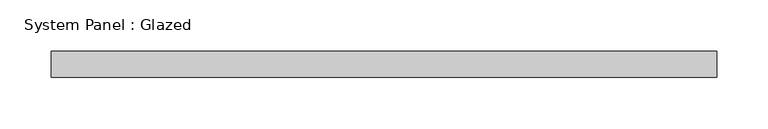
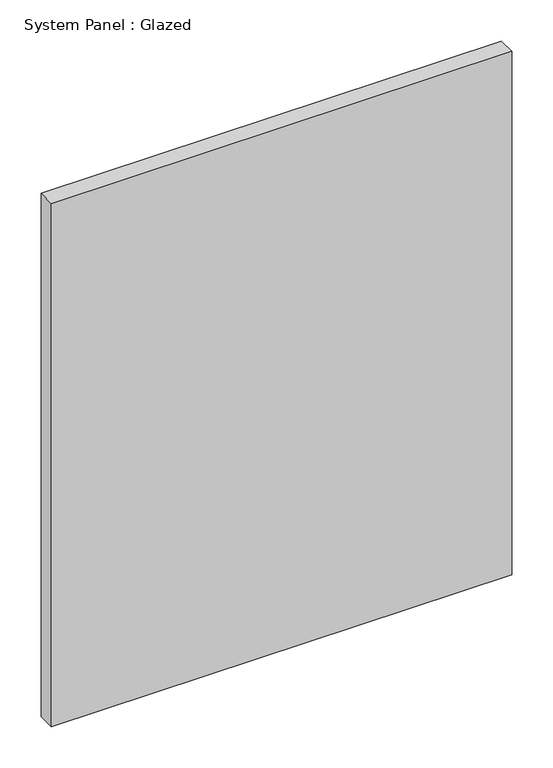
"""IFC4 building model written with IfcOpenShell, lengths in millimetres: plate geometry, System Panel : Glazed."""

from ifc_helpers import new_model, si_unit, origin, origin_with_axes, place, context, project, spatial, polyline, outline, extrude, source, transform, mapped, element, save


def system_panel_glazed_0ee6699b(model_context):
    return source(origin(), model_context, "Body", "SweptSolid", [
        extrude(outline(polyline([(323.85, 19.05), (-323.85, 19.05), (-323.85, 44.45), (323.85, 44.45), (323.85, 19.05)])), origin_with_axes(), (0.0, 0.0, 1.0), 778.3402035),
    ])


if __name__ == "__main__":
    model = new_model("IFC4")
    model_context = context("Model", 3, world=origin())
    ifc_project = project(units=[si_unit("LENGTHUNIT", "METRE", prefix="MILLI")], contexts=[model_context])
    site = spatial("IfcSite", under=ifc_project)
    building = spatial("IfcBuilding", under=site)
    placement = place(None, origin())
    system_panel_glazed_shape = system_panel_glazed_0ee6699b(model_context)
    element("IfcPlate", 1, ObjectType="System Panel : Glazed", at=placement, inside=building, context=model_context, shape_type="MappedRepresentation", body=[
        mapped(system_panel_glazed_shape, transform((0.0, 0.0, 0.0), x_axis=(1.0, 0.0, 0.0), y_axis=(0.0, 1.0, 0.0), z_axis=(0.0, 0.0, 1.0))),
    ])
    save(model, "model.ifc")

# Revit data of these elements
# Type "System Panel : Glazed"
#   Construction Type Id = "GSP4R"
#   Analytic Construction = "1/8 in Pilkington single glazing"
#   Visual Light Transmittance = 0.9
#   Solar Heat Gain Coefficient = 0.86
#   Heat Transfer Coefficient (U) = 1.18115 BTU/(h·ft²·°F)
#   Define Thermal Properties by = 1
# Element 1 (IfcPlate, "System Panel : Glazed")
#   Materials on its faces: "Glass"
# Materials
#   "Glass": class "Glass", colour RGB 0 128 192, transparency 0.75, Description = "Soda Lime Glass", Cost = 0
